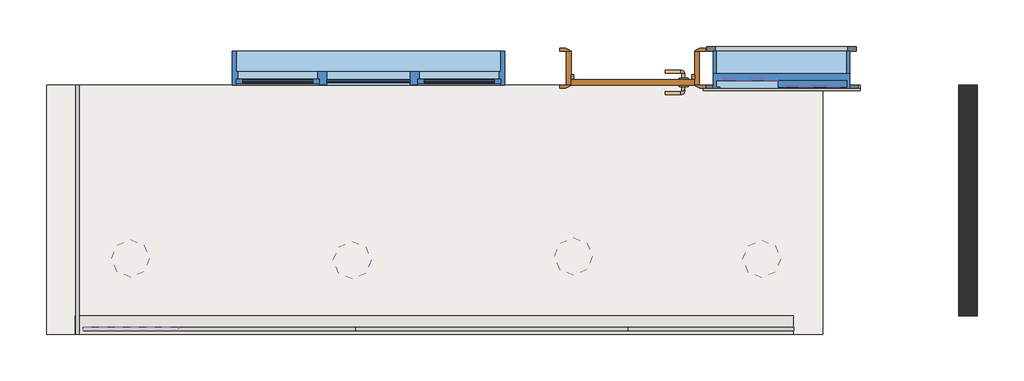
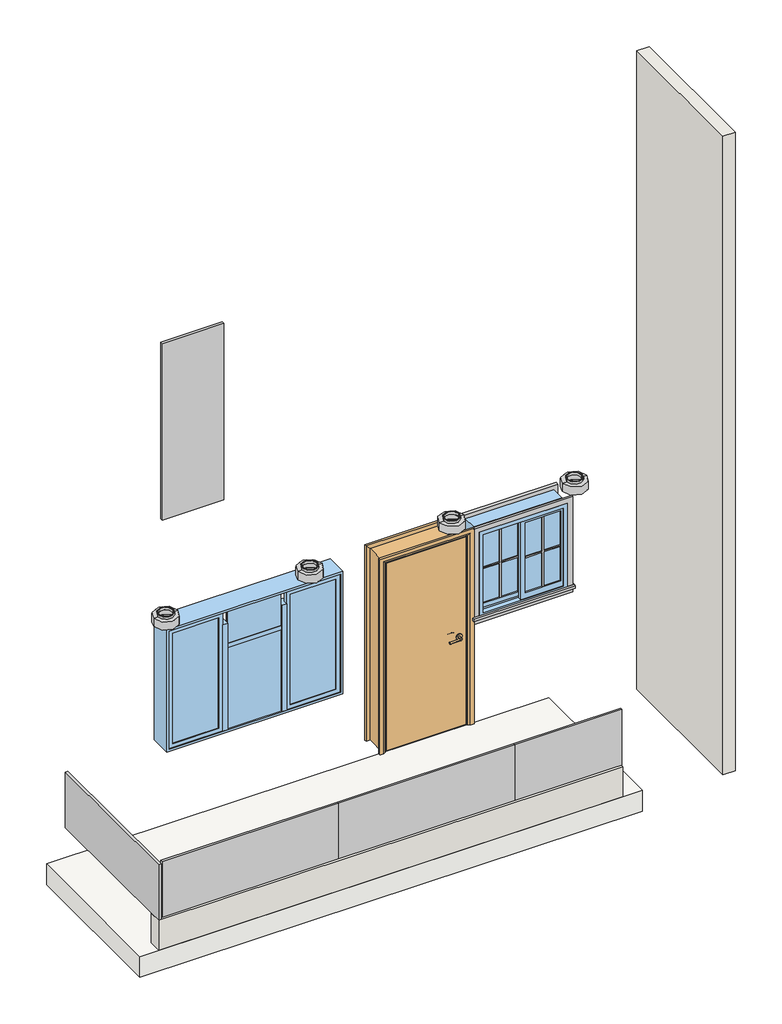
# One storey, incomplete: 5 plates, 4 light fixtures, 4 proxies, 2 walls, 2 windows, 1 door, 1 slab.
"""IFC4 building model written with IfcOpenShell, lengths in millimetres."""

from ifc_helpers import new_model, si_unit, frame, origin, place, context, project, spatial, polyline, outline, extrude, faceted_brep, transform, mapped, element, save
from components import muntin_pattern_2x2_muntin_pattern_2x2_5e7f5336, trim_window_exterior_flat_with_sill_84e24481, trim_window_interior_flat_picture_frame_28d4e5dc, doors_intsgl_910x2110mm_6866c2a0, ceiling_light_flat_round_60w_120v_7c4c2a52, system_panel_glazed_2daceabd, system_panel_glazed_5a474b37, system_panel_glazed_2ebb08bf, system_panel_glazed_678ad2c6, window_7a1f68bc, window_3ee5ce78

model = new_model("IFC4")

# Units and contexts
model_context = context("Model", 3, world=origin())
ifc_project = project(units=[si_unit("LENGTHUNIT", "METRE", prefix="MILLI")], contexts=[model_context])

# Site, building, storey
site = spatial("IfcSite", under=ifc_project)
building = spatial("IfcBuilding", under=site)
storey = spatial("IfcBuildingStorey", under=building, Elevation=4876.8)

# Proxies
placement = place(None, origin())
muntin_pattern_2x2_muntin_pattern_2x2_shape = muntin_pattern_2x2_muntin_pattern_2x2_5e7f5336(model_context)
element("IfcBuildingElementProxy", 1, Name="Muntin Pattern_2x2 : Muntin Pattern_2x2", ObjectType="Muntin Pattern_2x2 : Muntin Pattern_2x2", at=placement, inside=storey, context=model_context, shape_type="MappedRepresentation", body=[
    mapped(muntin_pattern_2x2_muntin_pattern_2x2_shape, transform((7924.3346961, -6872.0303244, 6126.1116728), x_axis=(-1.0, 0.0, 0.0), y_axis=(0.0, -1.0, 0.0), z_axis=(0.0, 0.0, 1.0))),
])
element("IfcBuildingElementProxy", 2, Name="Muntin Pattern_2x2 : Muntin Pattern_2x2", ObjectType="Muntin Pattern_2x2 : Muntin Pattern_2x2", at=placement, inside=storey, context=model_context, shape_type="MappedRepresentation", body=[
    mapped(muntin_pattern_2x2_muntin_pattern_2x2_shape, transform((8340.2596961, -6916.4803244, 6126.1116728), x_axis=(-1.0, 0.0, 0.0), y_axis=(0.0, -1.0, 0.0), z_axis=(0.0, 0.0, 1.0))),
])
trim_window_exterior_flat_with_sill_shape = trim_window_exterior_flat_with_sill_84e24481(model_context)
element("IfcBuildingElementProxy", 3, Name="Trim-Window-Exterior-Flat : with Sill", ObjectType="Trim-Window-Exterior-Flat : with Sill", at=placement, inside=storey, context=model_context, shape_type="MappedRepresentation", body=[
    mapped(trim_window_exterior_flat_with_sill_shape, transform((8132.2971961, -6926.0053244, 6957.9616728), x_axis=(1.0, 0.0, 0.0), y_axis=(0.0, 0.0, 1.0), z_axis=(0.0, -1.0, 0.0))),
])
trim_window_interior_flat_picture_frame_shape = trim_window_interior_flat_picture_frame_28d4e5dc(model_context)
element("IfcBuildingElementProxy", 4, Name="Trim-Window-Interior-Flat : Picture Frame", ObjectType="Trim-Window-Interior-Flat : Picture Frame", at=placement, inside=storey, context=model_context, shape_type="MappedRepresentation", body=[
    mapped(trim_window_interior_flat_picture_frame_shape, transform((8132.2971961, -6697.4053244, 6957.9616728), x_axis=(-1.0, 0.0, 0.0), y_axis=(0.0, 0.0, 1.0), z_axis=(0.0, 1.0, 0.0))),
])

# Door
doors_intsgl_910x2110mm_shape = doors_intsgl_910x2110mm_6866c2a0(model_context)
element("IfcDoor", 5, ObjectType="Doors_IntSgl : 910x2110mm", at=placement, inside=storey, context=model_context, shape_type="MappedRepresentation", body=[
    mapped(doors_intsgl_910x2110mm_shape, transform((7133.7935362, -6811.7053244, 4876.1169892), x_axis=(-1.0, 0.0, 0.0), y_axis=(0.0, -1.0, 0.0), z_axis=(0.0, 0.0, 1.0))),
])

# Light fixtures
ceiling_light_flat_round_60w_120v_shape = ceiling_light_flat_round_60w_120v_7c4c2a52(model_context)
element("IfcLightFixture", 6, ObjectType="Ceiling Light - Flat Round : 60W - 120V", at=placement, inside=storey, context=model_context, shape_type="MappedRepresentation", body=[
    mapped(ceiling_light_flat_round_60w_120v_shape, transform((3760.2328482, -8091.1180159, 5712.4203125), x_axis=(1.0, 0.0, 0.0), y_axis=(0.0, 1.0, 0.0), z_axis=(0.0, 0.0, 1.0))),
])
element("IfcLightFixture", 7, ObjectType="Ceiling Light - Flat Round : 60W - 120V", at=placement, inside=storey, context=model_context, shape_type="MappedRepresentation", body=[
    mapped(ceiling_light_flat_round_60w_120v_shape, transform((5248.5245352, -8102.6435841, 5712.4203125), x_axis=(1.0, 0.0, 0.0), y_axis=(0.0, 1.0, 0.0), z_axis=(0.0, 0.0, 1.0))),
])
element("IfcLightFixture", 8, ObjectType="Ceiling Light - Flat Round : 60W - 120V", at=placement, inside=storey, context=model_context, shape_type="MappedRepresentation", body=[
    mapped(ceiling_light_flat_round_60w_120v_shape, transform((6734.9014092, -8077.2504892, 5712.4203125), x_axis=(1.0, 0.0, 0.0), y_axis=(0.0, 1.0, 0.0), z_axis=(0.0, 0.0, 1.0))),
])
element("IfcLightFixture", 9, ObjectType="Ceiling Light - Flat Round : 60W - 120V", at=placement, inside=storey, context=model_context, shape_type="MappedRepresentation", body=[
    mapped(ceiling_light_flat_round_60w_120v_shape, transform((7999.6940621, -8094.5834343, 5712.4203125), x_axis=(1.0, 0.0, 0.0), y_axis=(0.0, 1.0, 0.0), z_axis=(0.0, 0.0, 1.0))),
])

# Plates
system_panel_glazed_shape = system_panel_glazed_2daceabd(model_context)
element("IfcPlate", 10, ObjectType="System Panel : Glazed", at=placement, inside=storey, context=model_context, shape_type="MappedRepresentation", body=[
    mapped(system_panel_glazed_shape, transform((4355.8722448, -8602.4053244, 5207.0), x_axis=(1.0, 0.0, 0.0), y_axis=(0.0, 1.0, 0.0), z_axis=(0.0, 0.0, 1.0))),
])
element("IfcPlate", 11, ObjectType="System Panel : Glazed", at=placement, inside=storey, context=model_context, shape_type="MappedRepresentation", body=[
    mapped(system_panel_glazed_shape, transform((6185.8722449, -8602.4053244, 5207.0), x_axis=(1.0, 0.0, 0.0), y_axis=(0.0, 1.0, 0.0), z_axis=(0.0, 0.0, 1.0))),
])
system_panel_glazed_2_shape = system_panel_glazed_5a474b37(model_context)
element("IfcPlate", 12, ObjectType="System Panel : Glazed", at=placement, inside=storey, context=model_context, shape_type="MappedRepresentation", body=[
    mapped(system_panel_glazed_2_shape, transform((3440.8722446, -7764.2053244, 5207.0), x_axis=(0.0, 1.0, 0.0), y_axis=(-1.0, 0.0, 0.0), z_axis=(0.0, 0.0, 1.0))),
])
system_panel_glazed_3_shape = system_panel_glazed_2ebb08bf(model_context)
element("IfcPlate", 13, ObjectType="System Panel : Glazed", at=placement, inside=storey, context=model_context, shape_type="MappedRepresentation", body=[
    mapped(system_panel_glazed_3_shape, transform((7657.1909411, -8602.4053244, 5207.0), x_axis=(1.0, 0.0, 0.0), y_axis=(0.0, 1.0, 0.0), z_axis=(0.0, 0.0, 1.0))),
])
system_panel_glazed_4_shape = system_panel_glazed_678ad2c6(model_context)
element("IfcPlate", 14, ObjectType="System Panel : Glazed", at=placement, inside=storey, context=model_context, shape_type="MappedRepresentation", body=[
    mapped(system_panel_glazed_4_shape, transform((3762.2223063, -8602.4053244, 9561.9327887), x_axis=(1.0, 0.0, 0.0), y_axis=(0.0, 1.0, 0.0), z_axis=(0.0, 0.0, 1.0))),
])

# Slab
element("IfcSlab", 15, ObjectType="9\"", at=placement, inside=storey, context=model_context, shape_type="SweptSolid", body=[
    extrude(outline(polyline([(8409.3004948, -6926.0053244), (8409.3004948, -8602.4053244), (3195.9504948, -8602.4053244), (3195.9504948, -6926.0053244), (8409.3004948, -6926.0053244)])), frame((0.0, 0.0, 4648.2), z_axis=(0.0, 0.0, 1.0), x_axis=(1.0, 0.0, 0.0)), (0.0, 0.0, 1.0), 228.6),
])

# Walls
element("IfcWall", 16, ObjectType="5\"", at=placement, inside=storey, context=model_context, shape_type="Brep", body=[
    faceted_brep([(3390.0722446, -8602.4053244, 4876.8), (8209.7222446, -8602.4053244, 4876.8), (8209.7222446, -8602.4053244, 5207.0), (3390.0722446, -8602.4053244, 5207.0), (3390.0722446, -8475.4053244, 4876.8), (3390.0722446, -8475.4053244, 5207.0), (3517.0722446, -8475.4053244, 5207.0), (8209.7222446, -8475.4053244, 5207.0), (8209.7222446, -8475.4053244, 4876.8), (3517.0722446, -8475.4053244, 4876.8)], [[[0, 1, 2, 3]], [[4, 5, 6, 7, 8, 9]], [[1, 0, 4, 9, 8]], [[2, 1, 8, 7]], [[3, 2, 7, 6, 5]], [[0, 3, 5, 4]]]),
])
element("IfcWall", 17, ObjectType="5\"", at=placement, inside=storey, context=model_context, shape_type="Brep", body=[
    faceted_brep([(9448.1305046, -8475.4053244, 4648.2), (9448.1305046, -8411.9053244, 4648.2), (9448.1305046, -6926.0053244, 4648.2), (9448.1305046, -6926.0053244, 11656.0203125), (9448.1305046, -8475.4053244, 11656.0203125), (9321.1305046, -6926.0053244, 4648.2), (9321.1305046, -8411.9053244, 4648.2), (9321.1305046, -8475.4053244, 4648.2), (9321.1305046, -8475.4053244, 11656.0203125), (9321.1305046, -6926.0053244, 11656.0203125)], [[[0, 1, 2, 3, 4]], [[5, 6, 7, 8, 9]], [[2, 1, 0, 7, 6, 5]], [[7, 0, 4, 8]], [[2, 5, 9, 3]], [[4, 3, 9, 8]]]),
])

# Windows
window_shape = window_7a1f68bc(model_context)
element("IfcWindow", 18, ObjectType="Window-Casement-Triple-Middle-Transom : 72\" x 53\"", at=placement, inside=storey, context=model_context, shape_type="MappedRepresentation", body=[
    mapped(window_shape, transform((5357.9935362, -6811.7053244, 4750.4881482), x_axis=(-1.0, 0.0, 0.0), y_axis=(0.0, -1.0, 0.0), z_axis=(0.0, 0.0, 1.0))),
])
window_2_shape = window_3ee5ce78(model_context)
element("IfcWindow", 19, ObjectType="Window-Sliding-Double : 36\" x 36\"", at=placement, inside=storey, context=model_context, shape_type="MappedRepresentation", body=[
    mapped(window_2_shape, transform((8132.2971961, -6815.5153244, 5129.1616728), x_axis=(-1.0, 0.0, 0.0), y_axis=(0.0, -1.0, 0.0), z_axis=(0.0, 0.0, 1.0))),
])

save(model, "model.ifc")

# Revit data of these elements
# Type "Muntin Pattern_2x2 : Muntin Pattern_2x2"
#   Width [instance default] = 4' - 0"
#   Thickness = 0' - 0 1/2"
#   Height [instance default] = 4' - 0"
#   Distance = 0' - 0 3/4"
#   Interior Material [instance default] = none
#   Exterior Material [instance default] = none
#   Default Elevation = 0
# Type "Trim-Window-Exterior-Flat : with Sill"
#   Trim Width = 0' - 2 1/4"
#   Trim Thickness_Picture Frame = 0' - 1 1/4"
#   Trim Thickness_with Sill = 0' - 0 3/4"
#   Sill Thickness = 0' - 1 1/4"
#   Opening Width [instance default] = 2' - 0"
#   Opening Height [instance default] = 3' - 0"
#   Default Elevation = 4' - 0"
#   Sill = yes
#   Picture Frame = no
#   Trim Material [instance default] = none
# Type "Trim-Window-Interior-Flat : Picture Frame"
#   Trim Thickness_Picture Frame = 0' - 1 1/4"
#   Trim Width = 0' - 2 1/4"
#   Trim Thickness_with Sill = 0' - 0 3/4"
#   Sill Thickness = 0' - 1 1/4"
#   Opening Width [instance default] = 2' - 0"
#   Opening Height [instance default] = 3' - 0"
#   Default Elevation = 4' - 0"
#   Sill = no
#   Picture Frame = yes
#   Trim Material [instance default] = none
# Type "Doors_IntSgl : 910x2110mm"
#   Construction Type Id = "MDOOR"
#   Type Mark = "41"
#   Type Comments = "Internal Single"
#   Operation = "SingleSwingRight"
#   Manufacturer = "Revit"
#   Keynote = "L20"
#   Description = "Internal Single Door"
#   Analytic Construction = "Metal"
#   UnderCut = 0' - 0.31496"
#   Tolerance = 0' - 0.07874"
#   Thickness = 0' - 1.49606"
#   Thermal Resistance (R) = 0.270117 (m²·K)/W
#   Structural Tolerance = 0' - 0.31496"
#   StopDepth = 0' - 1.25984"
#   Stop Thickness = 0' - 0.74803"
#   Rough Width = 2' - 11.82677"
#   Rough Height = 6' - 11.07087"
#   Height to Top Lock Rail = 3' - 3.37008"
#   Heat Transfer Coefficient (U) = 3.7021 W/(m²·K)
#   Handle Z Distance = 3' - 3.37008"
#   Handle X Distance = 0' - 2.95276"
#   Frame Thickness = 0' - 1.25984"
#   Door Panel Width = 2' - 8.51969"
#   Door Panel Thickness = 0' - 1.49606"
#   Door Panel Offset = 0' - 0"
#   Height = 6' - 11.07087"
#   Width = 2' - 11.82677"
#   Door Panel Height = 6' - 9.10236"
#   Architrave Setback = 0' - 0.19685"
#   Define Thermal Properties by = 1
#   Vis - Ironmongery = yes
#   Material Ironmongery = Door - Handle
#   Material Frame = Door - Frame/Mullion (1)
#   Material Door = Door - Panel
#   Material Architrave = Door - Architrave
#   Visual Light Transmittance = 0
#   Solar Heat Gain Coefficient = 0
#   Function = (empty or 0)
#   Wall Closure = (empty or 0)
# Type "Ceiling Light - Flat Round : 60W - 120V"
#   Lamp = "A-19"
#   Assembly Code = "D5020220"
#   Wattage = 60 W
#   built-in parameter 1150110 = 1 (stored number, unit not read)
#   built-in parameter 1114217 = 1 (stored number, unit not read)
#   built-in parameter 1150109 = 1 (stored number, unit not read)
#   built-in parameter 1150113 = 1 (stored number, unit not read)
#   built-in parameter 1150115 = 1 (stored number, unit not read)
#   built-in parameter 1150105 = 272.155 (stored number, unit not read)
#   Light Source Symbol Size = 2' - 0"
#   built-in parameter 1150112 = 1 (stored number, unit not read)
#   built-in parameter 1150114 = 1 (stored number, unit not read)
#   built-in parameter 1150107 = 2800 (stored number, unit not read)
#   built-in parameter 1150106 = 2.72155 (stored number, unit not read)
#   Emit from Circle Diameter = 0' - 10"
#   built-in parameter 1150104 = 1.32387 (stored number, unit not read)
#   Ballast Voltage = 120 V
#   built-in parameter 1114218 = 1 (stored number, unit not read)
#   built-in parameter 1150133 = 10 (stored number, unit not read)
#   Lumens = 855 lm
#   Apparent Load = 60 VA
#   built-in parameter 1150134 = 4
#   built-in parameter 1150137 = 1
#   Color Filter = 16777215
#   built-in parameter 1140040 [instance default] = 1
#   Ballast Number of Poles = 1
#   Light Box Material = Steel, Paint Finish, Dark Gray, Matte
#   Diffuser Material = Glass, White, High Luminance
#   Wattage Comments = ""
#   Emit Shape Visible in Rendering = no
#   Dimming Lamp Color Temperature Shift = (empty or 0)
#   Default Elevation = 0
# Type "System Panel : Glazed"
#   Keynote = "H11"
#   Construction Type Id = "GSP4R"
#   Analytic Construction = "1/8 in Pilkington single glazing"
#   Visual Light Transmittance = 0.9
#   Solar Heat Gain Coefficient = 0.86
#   Heat Transfer Coefficient (U) = 6.7069 W/(m²·K)
#   Define Thermal Properties by = 1
# Type "9\""
#   Keynote = "E60/130"
#   Function = 0
#   Layers, outside or top first: 0' - 9" "Concrete, Precast" (function 1)
# Type "5\""
#   Keynote = "F10"
#   Layers, outside or top first: 0' - 5" "Concrete" (function 1)
# Type "Window-Casement-Triple-Middle-Transom : 72\" x 53\""
#   Type Mark = "52"
#   Fire Rating = "0.5h"
#   Assembly Code = "B2020100"
#   Analytic Construction = "Double glazing - domestic"
#   Window Width = 2' - 0"
#   Window Inset [instance default] = 0' - 0 5/8"
#   Wall Thickness [instance default] = 0' - 6"
#   Visual Light Transmittance = 0.81
#   Transom Height Ratio = 0.3
#   Thermal Resistance (R) = 0.319569 (m²·K)/W
#   Solar Heat Gain Coefficient = 0.76
#   Rough Width = 6' - 0 1/2"
#   Rough Height = 4' - 5 1/2"
#   Heat Transfer Coefficient (U) = 3.12929 W/(m²·K)
#   Height = 4' - 5"
#   Transom Height = 1' - 3.9"
#   Frame Gap 3 [instance default] = 0' - 1 83/128"
#   Frame Gap 2 [instance default] = 0' - 0 5/8"
#   Frame Gap 1 = 0' - 1 51/128"
#   Default Sill Height = 3' - 0"
#   Width = 6' - 0"
#   Frame Material = Metal - Aluminum
#   Glass Panel Material = Glass
#   Wall Closure = (empty or 0)
# Type "Window-Sliding-Double : 36\" x 36\""
#   Type Mark = "51"
#   Fire Rating = "0.5h"
#   Assembly Code = "B2020100"
#   Analytic Construction = "Double glazing - domestic"
#   Window Inset [instance default] = 0' - 0"
#   Wall Thickness [instance default] = 0' - 6"
#   Visual Light Transmittance = 0.81
#   Thermal Resistance (R) = 0.319569 (m²·K)/W
#   Solar Heat Gain Coefficient = 0.76
#   Muntin Width = 1' - 2 5/8"
#   Muntin Height = 2' - 6 1/4"
#   Interior Wall Closure [instance default] = 0' - 2 3/4"
#   Heat Transfer Coefficient (U) = 3.12929 W/(m²·K)
#   Frame Extension [instance default] = 0' - 0 1/4"
#   Exterior Wall Closure [instance default] = 0' - 1 1/4"
#   Rough Width = 3' - 0 1/2"
#   Rough Height = 3' - 0 1/2"
#   Height = 3' - 0"
#   Extension Jamb [instance default] = 0' - 2 3/4"
#   Default Sill Height = 3' - 0"
#   Width = 3' - 0"
#   Interior Trim Visibility [instance default] = yes
#   Indicator Visibility [instance default] = yes
#   Exterior Trim Visibility [instance default] = yes
#   Muntin Visibility = yes
#   Extension Jamb Visibility [instance default] = yes
#   Muntin Pattern = Muntin Pattern_2x2 : Muntin Pattern_2x2
#   Interior Trim Material = Wood - Stained
#   Interior Trim = Trim-Window-Interior-Flat : Picture Frame
#   Interior Frame Material = Wood - Stained
#   Glass Panel Material = Glass
#   Exterior Trim Material = Clad - White
#   Exterior Trim = Trim-Window-Exterior-Flat : with Sill
#   Exterior Frame Material = Clad - White
#   Wall Closure = (empty or 0)
# Elements 1, 2 (IfcBuildingElementProxy, "Muntin Pattern_2x2 : Muntin Pattern_2x2")
#   Width = 1' - 2 5/8"
#   Height = 2' - 6 1/4"
#   Interior Material = Wood - Stained
#   Exterior Material = Clad - White
#   Phase Created = New Construction
#   Materials on its faces: "Clad - White", "Wood - Stained"
# Element 3 (IfcBuildingElementProxy, "Trim-Window-Exterior-Flat : with Sill")
#   Opening Width = 3' - 0"
#   Opening Height = 3' - 0"
#   Trim Material = Clad - White
#   Phase Created = New Construction
#   Materials on its faces: "Clad - White"
# Element 4 (IfcBuildingElementProxy, "Trim-Window-Interior-Flat : Picture Frame")
#   Opening Width = 3' - 0"
#   Opening Height = 3' - 0"
#   Trim Material = Wood - Stained
#   Phase Created = New Construction
#   Materials on its faces: "Wood - Stained"
# Element 5 (IfcDoor, "Doors_IntSgl : 910x2110mm")
#   Phase Created = New Construction
#   Materials on its faces: "Door - Architrave", "Door - Handle", "Door - Frame/Mullion (1)", "Door - Panel"
# Element 6 (IfcLightFixture, "Ceiling Light - Flat Round : 60W - 120V")
#   Mark = "12"
#   built-in parameter 1140040 = 1
#   Phase Created = New Construction
#   Materials on its faces: "Glass, White, High Luminance", "Steel, Paint Finish, Dark Gray, Matte"
# Element 7 (IfcLightFixture, "Ceiling Light - Flat Round : 60W - 120V")
#   Mark = "13"
#   built-in parameter 1140040 = 1
#   Phase Created = New Construction
#   Materials on its faces: "Glass, White, High Luminance", "Steel, Paint Finish, Dark Gray, Matte"
# Element 8 (IfcLightFixture, "Ceiling Light - Flat Round : 60W - 120V")
#   Mark = "14"
#   built-in parameter 1140040 = 1
#   Phase Created = New Construction
#   Materials on its faces: "Glass, White, High Luminance", "Steel, Paint Finish, Dark Gray, Matte"
# Element 9 (IfcLightFixture, "Ceiling Light - Flat Round : 60W - 120V")
#   Mark = "15"
#   built-in parameter 1140040 = 1
#   Phase Created = New Construction
#   Materials on its faces: "Glass, White, High Luminance", "Steel, Paint Finish, Dark Gray, Matte"
# Elements 10, 11, 12, 13, 14 (IfcPlate, "System Panel : Glazed")
#   Phase Created = New Construction
#   Materials on its faces: "Glass"
# Element 15 (IfcSlab, "9\"")
#   Height Offset From Level = 0' - 0"
#   Phase Created = New Construction
#   Materials on its faces: "Concrete, Precast"
# Element 16 (IfcWall, "5\"")
#   Top Offset = 0' - 0"
#   Base Offset = 0' - 0"
#   Unconnected Height = 1' - 1"
#   wall height = 1' - 1"
#   Phase Created = New Construction
#   Materials on its faces: "Concrete"
# Element 17 (IfcWall, "5\"")
#   built-in parameter 1001111 = -0' - 9"
#   Top Offset = 0' - 0"
#   Base Offset = -0' - 9"
#   Unconnected Height = 23' - 0"
#   wall height = 23' - 0"
#   Phase Created = New Construction
#   Materials on its faces: "Concrete", "Gypsum Wall Board"
# Element 18 (IfcWindow, "Window-Casement-Triple-Middle-Transom : 72\" x 53\"")
#   Mark = "4"
#   Window Inset = 0' - 0 5/8"
#   Frame Gap 3 = 0' - 1 83/128"
#   Frame Gap 2 = 0' - 0 5/8"
#   Phase Created = New Construction
#   Materials on its faces: "Metal - Aluminum", "Glass"
# Element 19 (IfcWindow, "Window-Sliding-Double : 36\" x 36\"")
#   Mark = "3"
#   Window Inset = 0' - 0"
#   Interior Wall Closure = 0' - 2 3/4"
#   Frame Extension = 0' - 0 1/4"
#   Exterior Wall Closure = 0' - 1 1/4"
#   Interior Trim Visibility = yes
#   Indicator Visibility = yes
#   Exterior Trim Visibility = yes
#   Phase Created = New Construction
#   Materials on its faces: "Wood - Stained", "Glass", "Clad - White"
# Materials
#   "Door - Handle": colour RGB 0 0 0, transparency 0, Keynote = "P21", Cost = 0
#   "Door - Frame/Mullion (1)": class "Wood", colour RGB 212 179 113, transparency 0, Keynote = "L20", Cost = 0
#   "Door - Panel": class "Wood", colour RGB 210 159 95, transparency 0, Keynote = "L20", Cost = 0
#   "Door - Architrave": class "Wood", colour RGB 154 90 5, transparency 0, Keynote = "P20", Cost = 0
#   "Steel, Paint Finish, Dark Gray, Matte": class "Metal", colour RGB 98 98 98, transparency 0, Description = "Steel, paint finish, dark gray, matte", Cost = 0
#   "Glass, White, High Luminance": class "Glass", colour RGB 249 250 249, transparency 0.8, Description = "physical material", Cost = 0
#   "Concrete, Precast": class "Concrete", colour RGB 192 192 192, transparency 0, Description = "Precast concrete", Cost = 0
#   "Concrete": class "Concrete", colour RGB 120 120 120, transparency 0, Description = "Portland Cement Concrete", Cost = 0
#   "Metal - Aluminum": class "Metal", colour RGB 247 247 247, transparency 0
#   "Glass": class "Glass", colour RGB 0 128 192, transparency 0.9, Description = "Soda Lime Glass", Cost = 0
#   "Wood - Stained": class "Wood", colour RGB 227 170 128, transparency 0, Cost = 0
#   "Clad - White": class "Wood", colour RGB 242 242 238, transparency 0, Cost = 0
#   "Gypsum Wall Board": class "Generic", colour RGB 249 249 249, transparency 0, Description = "Gypsum Wall Board", Cost = 0
